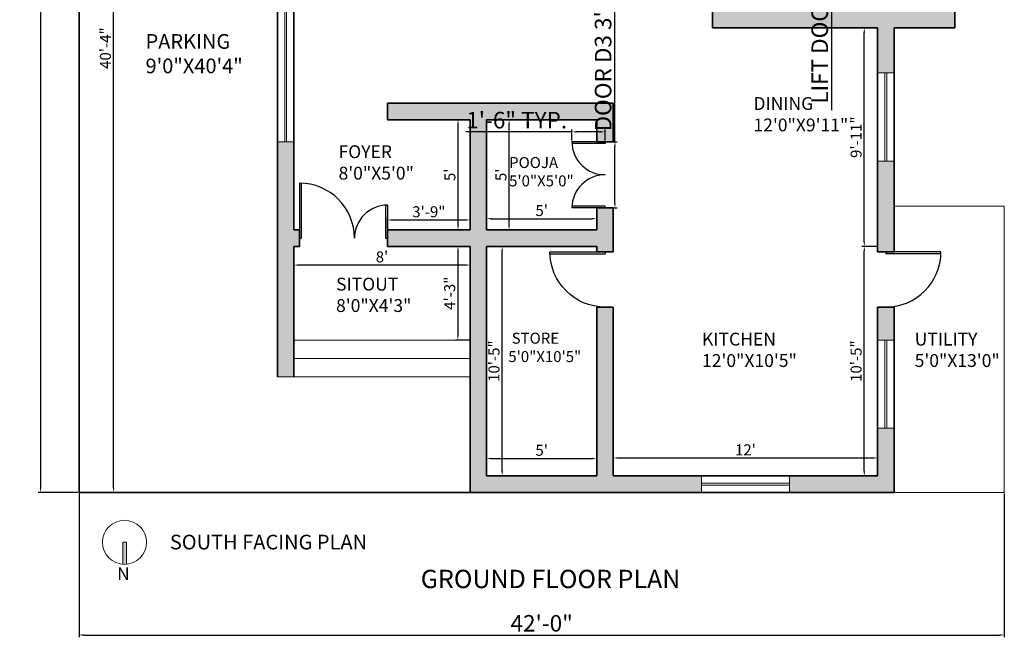
# Model space of a CAD drawing. Units: inches. Extents: x 4606 to 5879, y 1332 to 2209.
# Tile 5 of 7: x 5313 to 5849, y 1332 to 1669. Entities that reach past the tile are written whole.
import ezdxf

# ---------------------------------------------------------------- set-up
doc = ezdxf.new("R2010")
doc.units = ezdxf.units.IN
for name, color, linetype, lineweight in [('A-ANNO-DIMS', 2, 'Continuous', 18), ('A-ANNO-SYMB', 7, 'Continuous', 18), ('A-ANNO-TITL', 7, 'Continuous', 25), ('A-AREA-IDEN', 7, 'Continuous', 18), ('A-DOOR', 4, 'Continuous', 25), ('A-FLOR-PERI', 7, 'Continuous', 20), ('A-FLOR-STRS', 7, 'Continuous', 20), ('A-WALL', 7, 'Continuous', 35), ('A-WALL-PATT', 252, 'Continuous', 13), ('window', 130, 'Continuous', 18)]:
    doc.layers.add(name, color=color, linetype=linetype, lineweight=lineweight)
doc.styles.get("Standard").update_dxf_attribs({"font": 'arial.ttf'})
doc.dimstyles.new('ISO-25', dxfattribs={"dimtxt": 9, "dimasz": 2.5, "dimexe": 1.25, "dimexo": 0.625, "dimtad": 1, "dimlunit": 3, "dimtxsty": 'Standard', "dimcen": 2.5, "dimadec": 0, "dimazin": 0, "dimtfac": 1, "dimtmove": 0, "dimatfit": 3, "dimfxl": 1, "dimarcsym": 0})

# ---------------------------------------------------------------- blocks, each defined once
blk = doc.blocks.new('D')
for p, q in [((0, 30), (0, 0)), ((1, 29.93), (1, 0)), ((47, 18), (47, 0)), ((47, 18), (48, 18)), ((48, 18), (48, 0)), ((0, 0), (1, 0)), ((47, 0), (48, 0))]:
    blk.add_line(p, q)
for centre, radius, start, end in [((0, 0), 30, 0, 90), ((48, 0), 18, 90, 180)]:
    blk.add_arc(centre, radius, start, end)
blk = doc.blocks.new('D3')
for p, q in [((0, 0), (0, 18)), ((1, 0), (1, 18)), ((35, 0), (35, 18)), ((36, 0), (36, 18)), ((0, 0), (1, 0)), ((36, 0), (35, 0))]:
    blk.add_line(p, q)
for centre, start, end in [((0, 0), 0, 90), ((36, 0), 90, 180)]:
    blk.add_arc(centre, 18, start, end)
blk = doc.blocks.new('D2')
for p, q in [((0, 30), (0, 0)), ((1, 30), (1, 0)), ((0, 0), (1, 0))]:
    blk.add_line(p, q)
blk.add_arc((0, 0), 30, 0, 90)
blk = doc.blocks.new('*D26')
at = {"layer": 'A-ANNO-DIMS', "color": 0, "lineweight": -2, "transparency": 16777216}
for p, q in [((5344.24, 2081.24), (5322.61, 2081.24)), ((5323.86, 2078.74), (5323.86, 1413.74)), ((5344.24, 1411.24), (5322.61, 1411.24))]:
    blk.add_line(p, q, dxfattribs=at)
at = {"layer": 'A-ANNO-DIMS', "color": 0, "transparency": 16777216}
for points in [[(5323.44, 2078.74), (5324.28, 2078.74), (5323.86, 2081.24)], [(5323.44, 1413.74), (5324.28, 1413.74), (5323.86, 1411.24)]]:
    blk.add_solid(points, dxfattribs=at)
at = {"layer": 'Defpoints', "color": 0, "transparency": 16777216}
for p in [(5344.86, 2081.24), (5323.86, 1411.24), (5344.86, 1411.24)]:
    blk.add_point(p, dxfattribs=at)
at = {"layer": 'A-ANNO-DIMS', "color": 0, "transparency": 16777216, "insert": (5318.64, 1746.24), "char_height": 9, "attachment_point": 5, "rotation": 90}
blk.add_mtext('55\'-10"', dxfattribs=at)
blk = doc.blocks.new('*D42')
at = {"layer": 'A-ANNO-DIMS', "color": 0, "lineweight": -2, "transparency": 16777216}
for p, q in [((5635.86, 1420.86), (5635.86, 1431.28)), ((5638.36, 1430.03), (5777.36, 1430.03)), ((5779.86, 1420.86), (5779.86, 1431.28))]:
    blk.add_line(p, q, dxfattribs=at)
at = {"layer": 'A-ANNO-DIMS', "color": 0, "transparency": 16777216}
for points in [[(5638.36, 1430.44), (5638.36, 1429.61), (5635.86, 1430.03)], [(5777.36, 1430.44), (5777.36, 1429.61), (5779.86, 1430.03)]]:
    blk.add_solid(points, dxfattribs=at)
at = {"layer": 'Defpoints', "color": 0, "transparency": 16777216}
for p in [(5779.86, 1430.03), (5635.86, 1420.24), (5779.86, 1420.24)]:
    blk.add_point(p, dxfattribs=at)
at = {"layer": 'A-ANNO-DIMS', "color": 0, "transparency": 16777216, "insert": (5707.86, 1433.66), "char_height": 6, "attachment_point": 5}
blk.add_mtext("12'", dxfattribs=at)
blk = doc.blocks.new('*D43')
at = {"layer": 'A-ANNO-DIMS', "color": 0, "lineweight": -2, "transparency": 16777216}
for p, q in [((5567.49, 1545.24), (5576.59, 1545.24)), ((5575.34, 1422.74), (5575.34, 1542.74)), ((5567.49, 1420.24), (5576.59, 1420.24))]:
    blk.add_line(p, q, dxfattribs=at)
at = {"layer": 'A-ANNO-DIMS', "color": 0, "transparency": 16777216}
for points in [[(5574.92, 1542.74), (5575.76, 1542.74), (5575.34, 1545.24)], [(5574.92, 1422.74), (5575.76, 1422.74), (5575.34, 1420.24)]]:
    blk.add_solid(points, dxfattribs=at)
at = {"layer": 'Defpoints', "color": 0, "transparency": 16777216}
for p in [(5566.86, 1545.24), (5575.34, 1545.24), (5566.86, 1420.24)]:
    blk.add_point(p, dxfattribs=at)
at = {"layer": 'A-ANNO-DIMS', "color": 0, "transparency": 16777216, "insert": (5571.65, 1482.74), "char_height": 6, "attachment_point": 5, "rotation": 90}
blk.add_mtext('10\'-5"', dxfattribs=at)
blk = doc.blocks.new('*D44')
at = {"layer": 'A-ANNO-DIMS', "color": 0, "lineweight": -2, "transparency": 16777216}
for p, q in [((5566.86, 1420.86), (5566.86, 1430.97)), ((5569.36, 1429.72), (5624.36, 1429.72)), ((5626.86, 1420.86), (5626.86, 1430.97))]:
    blk.add_line(p, q, dxfattribs=at)
at = {"layer": 'A-ANNO-DIMS', "color": 0, "transparency": 16777216}
for points in [[(5569.36, 1430.14), (5569.36, 1429.3), (5566.86, 1429.72)], [(5624.36, 1430.14), (5624.36, 1429.3), (5626.86, 1429.72)]]:
    blk.add_solid(points, dxfattribs=at)
at = {"layer": 'Defpoints', "color": 0, "transparency": 16777216}
for p in [(5626.86, 1429.72), (5566.86, 1420.24), (5626.86, 1420.24)]:
    blk.add_point(p, dxfattribs=at)
at = {"layer": 'A-ANNO-DIMS', "color": 0, "transparency": 16777216, "insert": (5596.86, 1433.4), "char_height": 6, "attachment_point": 5}
blk.add_mtext("5'", dxfattribs=at)
blk = doc.blocks.new('*D45')
at = {"layer": 'A-ANNO-DIMS', "color": 0, "lineweight": -2, "transparency": 16777216}
for p, q in [((5567.49, 1614.24), (5580.35, 1614.24)), ((5579.1, 1556.74), (5579.1, 1611.74)), ((5567.49, 1554.24), (5580.35, 1554.24))]:
    blk.add_line(p, q, dxfattribs=at)
at = {"layer": 'A-ANNO-DIMS', "color": 0, "transparency": 16777216}
for points in [[(5578.69, 1611.74), (5579.52, 1611.74), (5579.1, 1614.24)], [(5578.69, 1556.74), (5579.52, 1556.74), (5579.1, 1554.24)]]:
    blk.add_solid(points, dxfattribs=at)
at = {"layer": 'Defpoints', "color": 0, "transparency": 16777216}
for p in [(5566.86, 1614.24), (5579.1, 1614.24), (5566.86, 1554.24)]:
    blk.add_point(p, dxfattribs=at)
at = {"layer": 'A-ANNO-DIMS', "color": 0, "transparency": 16777216, "insert": (5575.43, 1584.24), "char_height": 6, "attachment_point": 5, "rotation": 90}
blk.add_mtext("5'", dxfattribs=at)
blk = doc.blocks.new('*D46')
at = {"layer": 'A-ANNO-DIMS', "color": 0, "lineweight": -2, "transparency": 16777216}
for p, q in [((5557.24, 1614.24), (5550.05, 1614.24)), ((5551.3, 1556.74), (5551.3, 1611.74)), ((5557.24, 1554.24), (5550.05, 1554.24))]:
    blk.add_line(p, q, dxfattribs=at)
at = {"layer": 'A-ANNO-DIMS', "color": 0, "transparency": 16777216}
for points in [[(5550.88, 1611.74), (5551.71, 1611.74), (5551.3, 1614.24)], [(5550.88, 1556.74), (5551.71, 1556.74), (5551.3, 1554.24)]]:
    blk.add_solid(points, dxfattribs=at)
at = {"layer": 'Defpoints', "color": 0, "transparency": 16777216}
for p in [(5551.3, 1614.24), (5557.86, 1614.24), (5557.86, 1554.24)]:
    blk.add_point(p, dxfattribs=at)
at = {"layer": 'A-ANNO-DIMS', "color": 0, "transparency": 16777216, "insert": (5547.62, 1584.24), "char_height": 6, "attachment_point": 5, "rotation": 90}
blk.add_mtext("5'", dxfattribs=at)
blk = doc.blocks.new('*D47')
at = {"layer": 'A-ANNO-DIMS', "color": 0, "lineweight": -2, "transparency": 16777216}
for p, q in [((5512.86, 1554.86), (5512.86, 1560.91)), ((5557.86, 1554.86), (5557.86, 1560.91)), ((5515.36, 1559.66), (5555.36, 1559.66))]:
    blk.add_line(p, q, dxfattribs=at)
at = {"layer": 'A-ANNO-DIMS', "color": 0, "transparency": 16777216}
for points in [[(5515.36, 1560.07), (5515.36, 1559.24), (5512.86, 1559.66)], [(5555.36, 1560.07), (5555.36, 1559.24), (5557.86, 1559.66)]]:
    blk.add_solid(points, dxfattribs=at)
at = {"layer": 'Defpoints', "color": 0, "transparency": 16777216}
for p in [(5557.86, 1559.66), (5512.86, 1554.24), (5557.86, 1554.24)]:
    blk.add_point(p, dxfattribs=at)
at = {"layer": 'A-ANNO-DIMS', "color": 0, "transparency": 16777216, "insert": (5535.36, 1563.35), "char_height": 6, "attachment_point": 5}
blk.add_mtext('3\'-9"', dxfattribs=at)
blk = doc.blocks.new('*D48')
at = {"layer": 'A-ANNO-DIMS', "color": 0, "lineweight": -2, "transparency": 16777216}
for p, q in [((5566.86, 1554.86), (5566.86, 1561.58)), ((5626.86, 1554.86), (5626.86, 1561.58)), ((5569.36, 1560.33), (5624.36, 1560.33))]:
    blk.add_line(p, q, dxfattribs=at)
at = {"layer": 'A-ANNO-DIMS', "color": 0, "transparency": 16777216}
for points in [[(5569.36, 1560.75), (5569.36, 1559.92), (5566.86, 1560.33)], [(5624.36, 1560.75), (5624.36, 1559.92), (5626.86, 1560.33)]]:
    blk.add_solid(points, dxfattribs=at)
at = {"layer": 'Defpoints', "color": 0, "transparency": 16777216}
for p in [(5626.86, 1560.33), (5566.86, 1554.24), (5626.86, 1554.24)]:
    blk.add_point(p, dxfattribs=at)
at = {"layer": 'A-ANNO-DIMS', "color": 0, "transparency": 16777216, "insert": (5596.86, 1564.01), "char_height": 6, "attachment_point": 5}
blk.add_mtext("5'", dxfattribs=at)
blk = doc.blocks.new('*D53')
at = {"layer": 'A-ANNO-DIMS', "color": 0, "lineweight": -2, "transparency": 16777216}
for p, q in [((5779.24, 1545.24), (5771.33, 1545.24)), ((5772.58, 1422.74), (5772.58, 1542.74)), ((5779.24, 1420.24), (5771.33, 1420.24))]:
    blk.add_line(p, q, dxfattribs=at)
at = {"layer": 'A-ANNO-DIMS', "color": 0, "transparency": 16777216}
for points in [[(5772.16, 1542.74), (5773, 1542.74), (5772.58, 1545.24)], [(5772.16, 1422.74), (5773, 1422.74), (5772.58, 1420.24)]]:
    blk.add_solid(points, dxfattribs=at)
at = {"layer": 'Defpoints', "color": 0, "transparency": 16777216}
for p in [(5772.58, 1545.24), (5779.86, 1545.24), (5779.86, 1420.24)]:
    blk.add_point(p, dxfattribs=at)
at = {"layer": 'A-ANNO-DIMS', "color": 0, "transparency": 16777216, "insert": (5768.89, 1482.74), "char_height": 6, "attachment_point": 5, "rotation": 90}
blk.add_mtext('10\'-5"', dxfattribs=at)
blk = doc.blocks.new('*D54')
at = {"layer": 'A-ANNO-DIMS', "color": 0, "lineweight": -2, "transparency": 16777216}
for p, q in [((5773.2, 1664.24), (5773.83, 1664.24)), ((5772.58, 1547.74), (5772.58, 1661.74)), ((5779.24, 1545.24), (5771.33, 1545.24))]:
    blk.add_line(p, q, dxfattribs=at)
at = {"layer": 'A-ANNO-DIMS', "color": 0, "transparency": 16777216}
for points in [[(5772.16, 1661.74), (5773, 1661.74), (5772.58, 1664.24)], [(5772.16, 1547.74), (5773, 1547.74), (5772.58, 1545.24)]]:
    blk.add_solid(points, dxfattribs=at)
at = {"layer": 'Defpoints', "color": 0, "transparency": 16777216}
for p in [(5772.58, 1664.24), (5772.58, 1664.24), (5779.86, 1545.24)]:
    blk.add_point(p, dxfattribs=at)
at = {"layer": 'A-ANNO-DIMS', "color": 0, "transparency": 16777216, "insert": (5768.89, 1604.74), "char_height": 6, "attachment_point": 5, "rotation": 90}
blk.add_mtext('9\'-11"', dxfattribs=at)
blk = doc.blocks.new('*D55')
at = {"layer": 'A-ANNO-DIMS', "color": 0, "lineweight": -2, "transparency": 16777216}
for p, q in [((5557.24, 1545.24), (5549.96, 1545.24)), ((5551.21, 1542.74), (5551.21, 1496.74)), ((5557.24, 1494.24), (5549.96, 1494.24))]:
    blk.add_line(p, q, dxfattribs=at)
at = {"layer": 'A-ANNO-DIMS', "color": 0, "transparency": 16777216}
for points in [[(5550.8, 1542.74), (5551.63, 1542.74), (5551.21, 1545.24)], [(5550.8, 1496.74), (5551.63, 1496.74), (5551.21, 1494.24)]]:
    blk.add_solid(points, dxfattribs=at)
at = {"layer": 'Defpoints', "color": 0, "transparency": 16777216}
for p in [(5557.86, 1545.24), (5551.21, 1494.24), (5557.86, 1494.24)]:
    blk.add_point(p, dxfattribs=at)
at = {"layer": 'A-ANNO-DIMS', "color": 0, "transparency": 16777216, "insert": (5547.52, 1519.74), "char_height": 6, "attachment_point": 5, "rotation": 90}
blk.add_mtext('4\'-3"', dxfattribs=at)
blk = doc.blocks.new('*D56')
at = {"layer": 'A-ANNO-DIMS', "color": 0, "lineweight": -2, "transparency": 16777216}
for p, q in [((5461.86, 1544.61), (5461.86, 1533.83)), ((5557.86, 1544.61), (5557.86, 1533.83)), ((5555.36, 1535.08), (5464.36, 1535.08))]:
    blk.add_line(p, q, dxfattribs=at)
at = {"layer": 'A-ANNO-DIMS', "color": 0, "transparency": 16777216}
for points in [[(5464.36, 1535.49), (5464.36, 1534.66), (5461.86, 1535.08)], [(5555.36, 1535.49), (5555.36, 1534.66), (5557.86, 1535.08)]]:
    blk.add_solid(points, dxfattribs=at)
at = {"layer": 'Defpoints', "color": 0, "transparency": 16777216}
for p in [(5461.86, 1545.24), (5557.86, 1545.24), (5461.86, 1535.08)]:
    blk.add_point(p, dxfattribs=at)
at = {"layer": 'A-ANNO-DIMS', "color": 0, "transparency": 16777216, "insert": (5509.86, 1538.76), "char_height": 6, "attachment_point": 5}
blk.add_mtext("8'", dxfattribs=at)
blk = doc.blocks.new('*D57')
at = {"layer": 'A-ANNO-DIMS', "color": 0, "lineweight": -2, "transparency": 16777216}
for p, q in [((5345.49, 1895.24), (5364.92, 1895.24)), ((5363.67, 1413.74), (5363.67, 1892.74)), ((5345.49, 1411.24), (5364.92, 1411.24))]:
    blk.add_line(p, q, dxfattribs=at)
at = {"layer": 'A-ANNO-DIMS', "color": 0, "transparency": 16777216}
for points in [[(5363.25, 1892.74), (5364.08, 1892.74), (5363.67, 1895.24)], [(5363.25, 1413.74), (5364.08, 1413.74), (5363.67, 1411.24)]]:
    blk.add_solid(points, dxfattribs=at)
at = {"layer": 'Defpoints', "color": 0, "transparency": 16777216}
for p in [(5344.86, 1895.24), (5363.67, 1895.24), (5344.86, 1411.24)]:
    blk.add_point(p, dxfattribs=at)
at = {"layer": 'A-ANNO-DIMS', "color": 0, "transparency": 16777216, "insert": (5359.98, 1653.24), "char_height": 6, "attachment_point": 5, "rotation": 90}
blk.add_mtext('40\'-4"', dxfattribs=at)
blk = doc.blocks.new('GLAZING-72IN')
for p, q in [((0, 0), (0, 72)), ((1, 0), (1, 72))]:
    blk.add_line(p, q)
blk = doc.blocks.new('GLAZING-48IN')
for p, q in [((0, 0), (0, 48)), ((1, 0), (1, 48))]:
    blk.add_line(p, q)
blk = doc.blocks.new('NORTH-ARROW')
at = {"transparency": 33554687}
h = blk.add_hatch(color=256, dxfattribs=at)
h.dxf.hatch_style = 1
h.paths.add_polyline_path([(13, 20.5), (11, 20.5), (11, 8.55, 0.020861), (12, 8.5, 0.020861), (13, 8.55)])
for p, q in [((11, 8.5), (11, 20.5)), ((11, 20.5), (13, 20.5)), ((13, 20.5), (13, 8.55))]:
    blk.add_line(p, q)
blk.add_circle((12, 20.5), 12)
blk.add_text('N', height=6.9).set_placement((7.98, 0))
blk = doc.blocks.new('*D79')
at = {"layer": 'A-ANNO-DIMS', "color": 0, "lineweight": -2, "transparency": 16777216}
for p, q in [((5636.76, 1602.24), (5636.76, 1721.18)), ((5631.99, 1602.24), (5638.01, 1602.24)), ((5636.76, 1568.74), (5636.76, 1599.74)), ((5631.99, 1566.24), (5638.01, 1566.24))]:
    blk.add_line(p, q, dxfattribs=at)
at = {"layer": 'A-ANNO-DIMS', "color": 0, "transparency": 16777216}
for points in [[(5636.35, 1599.74), (5637.18, 1599.74), (5636.76, 1602.24)], [(5636.35, 1568.74), (5637.18, 1568.74), (5636.76, 1566.24)]]:
    blk.add_solid(points, dxfattribs=at)
at = {"layer": 'Defpoints', "color": 0, "transparency": 16777216}
for p in [(5631.36, 1602.24), (5636.76, 1602.24), (5631.36, 1566.24)]:
    blk.add_point(p, dxfattribs=at)
at = {"layer": 'A-ANNO-DIMS', "color": 0, "transparency": 16777216, "insert": (5631.48, 1662.96), "char_height": 9, "attachment_point": 5, "rotation": 90}
blk.add_mtext('DOOR D3 3\'-0" TYP.', dxfattribs=at)
blk = doc.blocks.new('*D80')
at = {"layer": 'A-ANNO-DIMS', "color": 0, "lineweight": -2, "transparency": 16777216}
for p, q in [((5613.36, 1607.64), (5555.6, 1607.64)), ((5613.36, 1602.86), (5613.36, 1608.89)), ((5628.86, 1607.64), (5615.86, 1607.64)), ((5631.36, 1602.86), (5631.36, 1608.89))]:
    blk.add_line(p, q, dxfattribs=at)
at = {"layer": 'A-ANNO-DIMS', "color": 0, "transparency": 16777216}
for points in [[(5615.86, 1608.06), (5615.86, 1607.22), (5613.36, 1607.64)], [(5628.86, 1608.06), (5628.86, 1607.22), (5631.36, 1607.64)]]:
    blk.add_solid(points, dxfattribs=at)
at = {"layer": 'Defpoints', "color": 0, "transparency": 16777216}
for p in [(5613.36, 1607.64), (5613.36, 1602.24), (5631.36, 1602.24)]:
    blk.add_point(p, dxfattribs=at)
at = {"layer": 'A-ANNO-DIMS', "color": 0, "transparency": 16777216, "insert": (5583.23, 1612.86), "char_height": 9, "attachment_point": 5}
blk.add_mtext('1\'-6" TYP.', dxfattribs=at)
blk = doc.blocks.new('*D81')
at = {"layer": 'A-ANNO-DIMS', "color": 0, "lineweight": -2, "transparency": 16777216}
for p, q in [((5749.99, 1784.24), (5756.01, 1784.24)), ((5754.76, 1781.74), (5754.76, 1750.74)), ((5749.99, 1748.24), (5756.01, 1748.24)), ((5754.76, 1748.24), (5754.76, 1619.48))]:
    blk.add_line(p, q, dxfattribs=at)
at = {"layer": 'A-ANNO-DIMS', "color": 0, "transparency": 16777216}
for points in [[(5754.35, 1781.74), (5755.18, 1781.74), (5754.76, 1784.24)], [(5754.35, 1750.74), (5755.18, 1750.74), (5754.76, 1748.24)]]:
    blk.add_solid(points, dxfattribs=at)
at = {"layer": 'Defpoints', "color": 0, "transparency": 16777216}
for p in [(5749.36, 1784.24), (5749.36, 1748.24), (5754.76, 1748.24)]:
    blk.add_point(p, dxfattribs=at)
at = {"layer": 'A-ANNO-DIMS', "color": 0, "transparency": 16777216, "insert": (5749.48, 1682.61), "char_height": 9, "attachment_point": 5, "rotation": 90}
blk.add_mtext('LIFT DOOR 3\'-0" TYP.', dxfattribs=at)
blk = doc.blocks.new('*D114')
at = {"layer": 'A-ANNO-DIMS', "color": 0, "lineweight": -2, "transparency": 16777216}
for p, q in [((5344.86, 1410.61), (5344.86, 1332.33)), ((5848.86, 1410.61), (5848.86, 1332.33)), ((5347.36, 1333.58), (5846.36, 1333.58))]:
    blk.add_line(p, q, dxfattribs=at)
at = {"layer": 'A-ANNO-DIMS', "color": 0, "transparency": 16777216}
for points in [[(5347.36, 1334), (5347.36, 1333.16), (5344.86, 1333.58)], [(5846.36, 1334), (5846.36, 1333.16), (5848.86, 1333.58)]]:
    blk.add_solid(points, dxfattribs=at)
at = {"layer": 'Defpoints', "color": 0, "transparency": 16777216}
for p in [(5344.86, 1411.24), (5848.86, 1411.24), (5848.86, 1333.58)]:
    blk.add_point(p, dxfattribs=at)
at = {"layer": 'A-ANNO-DIMS', "color": 0, "transparency": 16777216, "insert": (5596.86, 1338.8), "char_height": 9, "attachment_point": 5}
blk.add_mtext('42\'-0"', dxfattribs=at)

msp = doc.modelspace()

# ---------------------------------------------------------------- hatches: boundary and pattern name
at = {"layer": 'A-WALL-PATT', "transparency": 33554687}
h = msp.add_hatch(color=256, dxfattribs=at)
h.dxf.hatch_style = 1
h.paths.add_polyline_path([(5635.864, 1512.239), (5626.864, 1512.239), (5626.864, 1420.239), (5566.864, 1420.239), (5566.864, 1545.239), (5626.864, 1545.239), (5626.864, 1542.239), (5631.364, 1542.239), (5635.864, 1542.239), (5635.864, 1566.239), (5626.864, 1566.239), (5626.864, 1554.239), (5566.864, 1554.239), (5566.864, 1614.239), (5626.864, 1614.239), (5626.864, 1602.239), (5631.364, 1602.239), (5635.864, 1602.239), (5635.864, 1623.239), (5512.864, 1623.239), (5512.864, 1614.239), (5557.864, 1614.239), (5557.864, 1554.239), (5512.864, 1554.239), (5512.864, 1549.739), (5512.864, 1545.239), (5557.864, 1545.239), (5557.864, 1411.239), (5683.864, 1411.239), (5683.864, 1420.239), (5635.864, 1420.239)])
h.paths.add_polyline_path([(5788.864, 1446.239), (5779.864, 1446.239), (5779.864, 1420.239), (5731.864, 1420.239), (5731.864, 1411.239), (5788.864, 1411.239)])
h.paths.add_polyline_path([(5788.864, 1512.239), (5779.864, 1512.239), (5779.864, 1494.239), (5788.864, 1494.239)])
h.paths.add_polyline_path([(5788.864, 1591.739), (5779.864, 1591.739), (5779.864, 1542.239), (5788.864, 1542.239)])
h.paths.add_polyline_path([(5821.864, 1691.239), (5812.864, 1691.239), (5812.864, 1673.239), (5716.864, 1673.239), (5716.864, 1676.239), (5712.364, 1676.239), (5707.864, 1676.239), (5707.864, 1673.239), (5689.864, 1673.239), (5689.864, 1664.239), (5779.864, 1664.239), (5779.864, 1639.739), (5788.864, 1639.739), (5788.864, 1664.239), (5821.864, 1664.239)])
h.paths.add_polyline_path([(5821.864, 1823.239), (5812.864, 1823.239), (5812.864, 1799.239), (5714.864, 1799.239), (5714.864, 1790.239), (5743.864, 1790.239), (5743.864, 1784.239), (5752.864, 1784.239), (5752.864, 1790.239), (5812.864, 1790.239), (5812.864, 1742.239), (5752.864, 1742.239), (5752.864, 1748.239), (5743.864, 1748.239), (5743.864, 1742.239), (5707.864, 1742.239), (5707.864, 1706.239), (5716.864, 1706.239), (5716.864, 1733.239), (5812.864, 1733.239), (5812.864, 1715.239), (5821.864, 1715.239)])
h.paths.add_polyline_path([(5821.864, 1928.239), (5812.864, 1928.239), (5812.864, 1904.239), (5713.864, 1904.239), (5713.864, 1895.239), (5812.864, 1895.239), (5812.864, 1871.239), (5821.864, 1871.239)])
h.paths.add_polyline_path([(5821.864, 2006.239), (5812.864, 2006.239), (5812.864, 1976.239), (5821.864, 1976.239)])
h.paths.add_polyline_path([(5821.864, 2081.239), (5779.864, 2081.239), (5779.864, 2072.239), (5812.864, 2072.239), (5812.864, 2054.239), (5821.864, 2054.239)])
h.paths.add_polyline_path([(5707.864, 2081.239), (5650.864, 2081.239), (5650.864, 2072.239), (5668.864, 2072.239), (5668.864, 1976.239), (5662.864, 1976.239), (5662.864, 1970.239), (5668.864, 1970.239), (5668.864, 1955.239), (5674.864, 1955.239), (5674.864, 2072.239), (5707.864, 2072.239)])
h.paths.add_polyline_path([(5626.864, 2081.239), (5578.864, 2081.239), (5578.864, 2072.239), (5602.864, 2072.239), (5602.864, 1976.239), (5566.864, 1976.239), (5566.864, 1970.239), (5602.864, 1970.239), (5602.864, 1904.239), (5530.864, 1904.239), (5530.864, 1925.239), (5521.864, 1925.239), (5521.864, 1904.239), (5518.864, 1904.239), (5518.864, 1895.239), (5605.864, 1895.239), (5677.864, 1895.239), (5677.864, 1904.239), (5674.864, 1904.239), (5674.864, 1925.239), (5668.864, 1925.239), (5668.864, 1904.239), (5608.864, 1904.239), (5608.864, 1970.239), (5632.864, 1970.239), (5632.864, 1976.239), (5608.864, 1976.239), (5608.864, 2072.239), (5626.864, 2072.239)])
h.paths.add_polyline_path([(5554.864, 2081.239), (5473.864, 2081.239), (5473.864, 2072.239), (5521.864, 2072.239), (5521.864, 1955.239), (5530.864, 1955.239), (5530.864, 1970.239), (5536.864, 1970.239), (5536.864, 1976.239), (5530.864, 1976.239), (5530.864, 2072.239), (5554.864, 2072.239)])
h.paths.add_polyline_path([(5401.864, 2081.239), (5344.864, 2081.239), (5344.864, 2054.239), (5353.864, 2054.239), (5353.864, 2072.239), (5401.864, 2072.239)])
h.paths.add_polyline_path([(5353.864, 2006.239), (5344.864, 2006.239), (5344.864, 1970.239), (5353.864, 1970.239)])
h.paths.add_polyline_path([(5482.864, 1904.239), (5353.864, 1904.239), (5353.864, 1922.239), (5344.864, 1922.239), (5344.864, 1895.239), (5452.864, 1895.239), (5452.864, 1674.239), (5461.864, 1674.239), (5461.864, 1895.239), (5482.864, 1895.239)])
h.paths.add_polyline_path([(5461.864, 1602.239), (5452.864, 1602.239), (5452.864, 1474.239), (5461.864, 1474.239), (5461.864, 1545.239), (5464.864, 1545.239), (5464.864, 1554.239), (5461.864, 1554.239)])

# ---------------------------------------------------------------- linework, layer by layer
at = {"layer": 'A-FLOR-PERI'}
for p, q in [((5848.864, 1567.239), (5788.864, 1567.239)), ((5848.864, 1411.239), (5848.864, 1567.239)), ((5788.864, 1411.239), (5848.864, 1411.239))]:
    msp.add_line(p, q, dxfattribs=at)
at = {"layer": 'A-FLOR-STRS'}
for p, q in [((5461.864, 1494.239), (5557.864, 1494.239)), ((5461.864, 1484.239), (5557.864, 1484.239)), ((5452.864, 1474.239), (5557.864, 1474.239))]:
    msp.add_line(p, q, dxfattribs=at)
at = {"layer": 'A-WALL'}
for p, q in [((5452.864, 1895.239), (5452.864, 1474.239)), ((5461.864, 1895.239), (5461.864, 1554.239)), ((5689.864, 1664.239), (5689.864, 1673.239)), ((5779.864, 1664.239), (5689.864, 1664.239)), ((5779.864, 1664.239), (5779.864, 1542.239)), ((5821.864, 1664.239), (5788.864, 1664.239)), ((5788.864, 1664.239), (5788.864, 1542.239)), ((5512.864, 1623.239), (5512.864, 1614.239)), ((5635.864, 1623.239), (5512.864, 1623.239)), ((5635.864, 1623.239), (5635.864, 1602.239)), ((5512.864, 1614.239), (5557.864, 1614.239)), ((5557.864, 1614.239), (5557.864, 1554.239)), ((5566.864, 1614.239), (5626.864, 1614.239)), ((5566.864, 1614.239), (5566.864, 1554.239)), ((5626.864, 1614.239), (5626.864, 1602.239)), ((5626.864, 1602.239), (5635.864, 1602.239)), ((5626.864, 1566.239), (5635.864, 1566.239)), ((5626.864, 1566.239), (5626.864, 1554.239)), ((5635.864, 1566.239), (5635.864, 1542.239)), ((5461.864, 1554.239), (5464.864, 1554.239)), ((5464.864, 1554.239), (5464.864, 1545.239)), ((5512.864, 1554.239), (5557.864, 1554.239)), ((5512.864, 1554.239), (5512.864, 1545.239)), ((5566.864, 1554.239), (5626.864, 1554.239)), ((5461.864, 1545.239), (5464.864, 1545.239)), ((5461.864, 1545.239), (5461.864, 1474.239)), ((5512.864, 1545.239), (5557.864, 1545.239)), ((5557.864, 1545.239), (5557.864, 1411.239)), ((5566.864, 1545.239), (5626.864, 1545.239)), ((5566.864, 1545.239), (5566.864, 1420.239)), ((5626.864, 1545.239), (5626.864, 1542.239)), ((5626.864, 1542.239), (5635.864, 1542.239)), ((5779.864, 1542.239), (5788.864, 1542.239)), ((5626.864, 1512.239), (5635.864, 1512.239)), ((5626.864, 1512.239), (5626.864, 1420.239)), ((5635.864, 1512.239), (5635.864, 1420.239)), ((5779.864, 1512.239), (5779.864, 1420.239)), ((5779.864, 1512.239), (5788.864, 1512.239)), ((5788.864, 1512.239), (5788.864, 1411.239)), ((5566.864, 1420.239), (5626.864, 1420.239)), ((5635.864, 1420.239), (5779.864, 1420.239))]:
    msp.add_line(p, q, dxfattribs=at)
msp.add_lwpolyline([(5821.864, 1664.239), (5821.864, 2081.239), (5344.864, 2081.239), (5344.864, 1411.239), (5788.864, 1411.239)], dxfattribs=at)
at = {"layer": 'window'}
for p, q in [((5779.864, 1639.739), (5788.864, 1639.739)), ((5452.864, 1602.239), (5461.864, 1602.239)), ((5779.864, 1591.739), (5788.864, 1591.739)), ((5779.864, 1494.239), (5788.864, 1494.239)), ((5779.864, 1446.239), (5788.864, 1446.239)), ((5683.864, 1420.239), (5683.864, 1411.239)), ((5731.864, 1420.239), (5731.864, 1411.239))]:
    msp.add_line(p, q, dxfattribs=at)

# ---------------------------------------------------------------- block references
at = {"layer": 'A-ANNO-SYMB'}
msp.add_blockref('NORTH-ARROW', (5357.613, 1363.576), dxfattribs=at)
at = {"layer": 'A-DOOR'}
for name, p, rotation in [('D3', (5631.364, 1566.239), 90), ('D2', (5784.364, 1542.239), 270)]:
    msp.add_blockref(name, p, dxfattribs=dict(at, rotation=rotation))
msp.add_blockref('D', (5464.864, 1549.739), dxfattribs=at)
at = {"layer": 'A-DOOR', "xscale": -1, "rotation": 90}
msp.add_blockref('D2', (5631.364, 1542.239), dxfattribs=at)
at = {"layer": 'window'}
for name, p in [('GLAZING-72IN', (5456.864, 1602.239)), ('GLAZING-48IN', (5783.864, 1591.739)), ('GLAZING-48IN', (5783.864, 1446.239))]:
    msp.add_blockref(name, p, dxfattribs=at)
at = {"layer": 'window', "rotation": 270.0000000000001}
msp.add_blockref('GLAZING-48IN', (5683.865, 1416.239), dxfattribs=at)

# ---------------------------------------------------------------- texts
at = {"layer": 'A-ANNO-TITL', "attachment_point": 1}
for s, insert, char_height in [('{\\fTimes New Roman|b0|i0|c0|p18;SOUTH FACING PLAN}', (5394.307, 1388.203), 8), ('{\\fTimes New Roman|b0|i0|c0|p18;GROUND FLOOR PLAN}', (5530.954, 1369.116), 10)]:
    msp.add_mtext_dynamic_manual_height_columns(s, width=196.26071, gutter_width=12.5, heights=[0], dxfattribs=dict(at, insert=insert, char_height=char_height))
at = {"layer": 'A-AREA-IDEN', "attachment_point": 1}
for s, width, insert, char_height in [('{\\fTimes New Roman|b0|i0|c0|p18;PARKING\\P9\'0"X40\'4"}', 110.76054, (5381.062, 1660.892), 8), ('{\\fTimes New Roman|b0|i0|c0|p18;DINING\\P12\'0"X9\'11"}', 80.30411, (5712.226, 1626.577), 7), ('{\\fTimes New Roman|b0|i0|c0|p18;FOYER\\P8\'0"X5\'0"}', 80.30411, (5486.209, 1600.32), 7), ('{\\fTimes New Roman|b0|i0|c0|p18;POOJA\\P5\'0"X5\'0"}', 80.30411, (5579.102, 1593.934), 6), ('{\\fTimes New Roman|b0|i0|c0|p18;SITOUT\\P8\'0"X4\'3"}', 80.30411, (5484.86, 1528.201), 7), ('{\\fTimes New Roman|b0|i0|c0|p18; STORE\\P5\'0"X10\'5"}', 80.30411, (5578.67, 1498.248), 6), ('{\\fTimes New Roman|b0|i0|c0|p18;KITCHEN\\P12\'0"X10\'5"}', 80.30411, (5684.209, 1498.248), 7), ('{\\fTimes New Roman|b0|i0|c0|p18;UTILITY\\P5\'0"X13\'0"}', 80.30411, (5800.041, 1498.248), 7)]:
    msp.add_mtext_dynamic_manual_height_columns(s, width=width, gutter_width=12.5, heights=[0], dxfattribs=dict(at, insert=insert, char_height=char_height))

# ---------------------------------------------------------------- dimensions: what is measured, and where the dimension line sits
at = {"layer": 'A-ANNO-DIMS'}
for base, p1, p2, angle, override, picture, middle in [((5323.86, 1411.239), (5344.864, 2081.239), (5344.864, 1411.239), 90, {"dimclrd": 0, "dimclre": 0, "dimclrt": 0}, '*D26', (5318.639, 1746.239)), ((5363.666, 1895.239), (5344.864, 1411.239), (5344.864, 1895.239), 90, {"dimtxt": 6, "dimclrd": 0, "dimclre": 0, "dimclrt": 0}, '*D57', (5359.977, 1653.239)), ((5772.578, 1664.239), (5779.864, 1545.239), (5772.578, 1664.239), 90, {"dimtxt": 6, "dimclrd": 0, "dimclre": 0, "dimclrt": 0, "dimtmove": 1}, '*D54', (5768.89, 1604.739)), ((5551.295, 1614.239), (5557.864, 1554.239), (5557.864, 1614.239), 270, {"dimtxt": 6, "dimclrd": 0, "dimclre": 0, "dimclrt": 0}, '*D46', (5547.619, 1584.239)), ((5579.102, 1614.239), (5566.864, 1554.239), (5566.864, 1614.239), 270, {"dimtxt": 6, "dimclrd": 0, "dimclre": 0, "dimclrt": 0}, '*D45', (5575.426, 1584.239)), ((5551.215, 1494.239), (5557.864, 1545.239), (5557.864, 1494.239), 90, {"dimtxt": 6, "dimclrd": 0, "dimclre": 0, "dimclrt": 0}, '*D55', (5547.524, 1519.739)), ((5575.339, 1545.239), (5566.864, 1420.239), (5566.864, 1545.239), 270, {"dimtxt": 6, "dimclrd": 0, "dimclre": 0, "dimclrt": 0}, '*D43', (5571.651, 1482.739)), ((5772.578, 1545.239), (5779.864, 1420.239), (5779.864, 1545.239), 90, {"dimtxt": 6, "dimclrd": 0, "dimclre": 0, "dimclrt": 0}, '*D53', (5768.89, 1482.739))]:
    dim = msp.add_linear_dim(base=base, p1=p1, p2=p2, angle=angle, dimstyle='ISO-25', override=override, dxfattribs=at)
    dim.commit()
    dim.dimension.update_dxf_attribs({"geometry": picture, "text_midpoint": middle})
for base, p1, p2, angle, text, picture, middle in [((5754.764, 1748.239), (5749.364, 1784.239), (5749.364, 1748.239), 270, 'LIFT DOOR <> TYP.', '*D81', (5749.48, 1682.608)), ((5636.764, 1602.239), (5631.364, 1566.239), (5631.364, 1602.239), 90, 'DOOR D3 <> TYP.', '*D79', (5631.48, 1662.958)), ((5613.364, 1607.639), (5631.364, 1602.239), (5613.364, 1602.239), 180, '<> TYP.', '*D80', (5583.233, 1612.859))]:
    dim = msp.add_linear_dim(base=base, p1=p1, p2=p2, angle=angle, text=text, dimstyle='ISO-25', override={"dimdec": 1, "dimlfac": 1, "dimrnd": 0, "dimzin": 1, "dimdsep": 46, "dimlunit": 4, "dimfrac": 2}, dxfattribs=at)
    dim.commit()
    dim.dimension.update_dxf_attribs({"geometry": picture, "text_midpoint": middle})
for base, p1, p2, override, picture, middle in [((5557.864, 1559.655), (5512.864, 1554.239), (5557.864, 1554.239), {"dimtxt": 6, "dimclrd": 0, "dimclre": 0, "dimclrt": 0}, '*D47', (5535.364, 1563.346)), ((5626.864, 1560.332), (5566.864, 1554.239), (5626.864, 1554.239), {"dimtxt": 6, "dimclrd": 0, "dimclre": 0, "dimclrt": 0}, '*D48', (5596.864, 1564.008)), ((5461.864, 1535.077), (5557.864, 1545.239), (5461.864, 1545.239), {"dimtxt": 6, "dimclrd": 0, "dimclre": 0, "dimclrt": 0}, '*D56', (5509.864, 1538.765)), ((5626.864, 1429.719), (5566.864, 1420.239), (5626.864, 1420.239), {"dimtxt": 6, "dimclrd": 0, "dimclre": 0, "dimclrt": 0}, '*D44', (5596.864, 1433.395)), ((5779.864, 1430.027), (5635.864, 1420.239), (5779.864, 1420.239), {"dimtxt": 6, "dimclrd": 0, "dimclre": 0, "dimclrt": 0}, '*D42', (5707.864, 1433.664)), ((5848.864, 1333.58), (5344.864, 1411.239), (5848.864, 1411.239), {"dimdec": 1, "dimlfac": 1, "dimrnd": 0, "dimzin": 1, "dimdsep": 46, "dimlunit": 4, "dimfrac": 2}, '*D114', (5596.864, 1338.8))]:
    dim = msp.add_linear_dim(base=base, p1=p1, p2=p2, dimstyle='ISO-25', override=override, dxfattribs=at)
    dim.commit()
    dim.dimension.update_dxf_attribs({"geometry": picture, "text_midpoint": middle})

doc.saveas('drawing.dxf')
